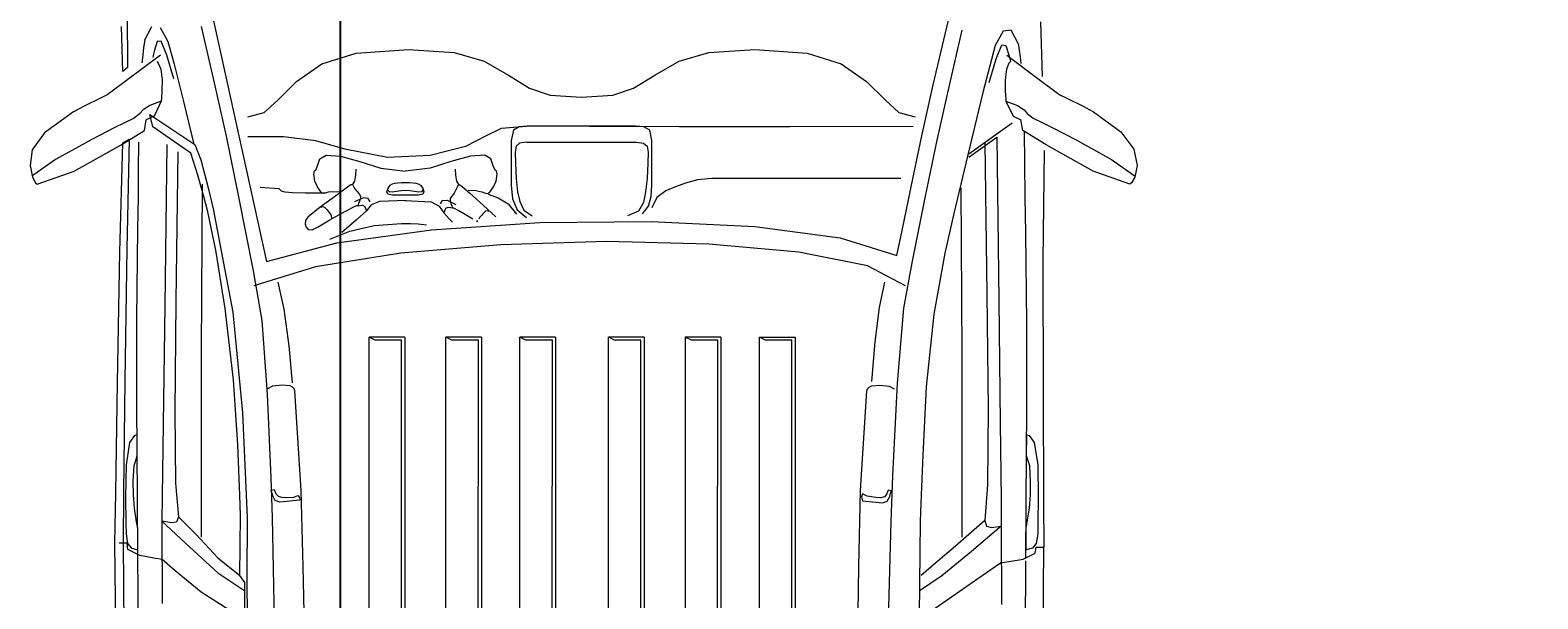
# Model space of a CAD drawing. Units: inches. Extents: x -4347 to -3836, y 955 to 1521.
# Tile 4 of 11: x -4133 to -4072, y 1065 to 1088. Entities that reach past the tile are written whole.
import ezdxf

# ---------------------------------------------------------------- set-up
doc = ezdxf.new("R2010")
doc.units = ezdxf.units.IN
doc.header["$MEASUREMENT"] = 0
doc.layers.add('A-ANNO-DIMS', color=2, linetype='Continuous', lineweight=18)
doc.layers.add('A-SITE-VEHC', color=8, linetype='Continuous', lineweight=13)
doc.styles.get("Standard").update_dxf_attribs({"font": 'arial.ttf'})
doc.dimstyles.get("Standard").update_dxf_attribs({"dimtxt": 0.18, "dimasz": 0.18, "dimexe": 0.18, "dimexo": 0.0625, "dimgap": 0.09, "dimtad": 0, "dimtih": 1, "dimtoh": 1, "dimdec": 0, "dimzin": 0, "dimdsep": 46, "dimlunit": 3, "dimtxsty": 'Standard', "dimcen": 0.09, "dimadec": 0, "dimazin": 0, "dimtfac": 1, "dimtdec": 0, "dimtofl": 0, "dimtmove": 0, "dimatfit": 3, "dimfxl": 1, "dimtolj": 1, "dimtzin": 0, "dimarcsym": 0})

# ---------------------------------------------------------------- blocks, each defined once
blk = doc.blocks.new('*D47')
at = {"layer": 'A-ANNO-DIMS', "color": 0, "lineweight": -2, "transparency": 16777216}
for p, q in [((-4120.58, 1288.726), (-4120.58, 966.959)), ((-3940.58, 1288.726), (-3940.58, 966.959)), ((-4120.4, 967.139), (-4030.97, 967.139)), ((-3940.76, 967.139), (-4030.189, 967.139))]:
    blk.add_line(p, q, dxfattribs=at)
at = {"layer": 'A-ANNO-DIMS', "color": 0, "transparency": 16777216}
for points in [[(-4120.4, 967.169), (-4120.4, 967.109), (-4120.58, 967.139)], [(-3940.76, 967.169), (-3940.76, 967.109), (-3940.58, 967.139)]]:
    blk.add_solid(points, dxfattribs=at)
at = {"layer": 'Defpoints', "color": 0, "transparency": 16777216}
for p in [(-4120.58, 1288.789), (-3940.58, 1288.789), (-3940.58, 967.139)]:
    blk.add_point(p, dxfattribs=at)
at = {"layer": 'A-ANNO-DIMS', "color": 0, "transparency": 16777216, "insert": (-4030.58, 967.139), "char_height": 0.18, "attachment_point": 5}
blk.add_mtext('\\A1;15\'-0"', dxfattribs=at)

msp = doc.modelspace()

# ---------------------------------------------------------------- linework, layer by layer
at = {"layer": 'A-SITE-VEHC'}
for p, q in [((-4125.796, 1088.55), (-4123.555, 1078.317)), ((-4096.245, 1087.523), (-4096.02, 1088.485)), ((-4129.327, 1085.96), (-4129.374, 1087.772)), ((-4129.151, 1088.327), (-4129.134, 1086.126)), ((-4128.446, 1087.238), (-4128.158, 1087.781)), ((-4126.173, 1087.783), (-4125.652, 1085.508)), ((-4092.424, 1087.964), (-4092.357, 1085.761)), ((-4128.446, 1087.238), (-4128.489, 1086.935)), ((-4127.947, 1087.167), (-4128.057, 1086.827)), ((-4127.78, 1087.191), (-4127.947, 1087.167)), ((-4127.831, 1087.739), (-4127.52, 1087.167)), ((-4127.557, 1086.621), (-4127.78, 1087.191)), ((-4127.52, 1087.167), (-4127.264, 1086.261)), ((-4096.732, 1085.425), (-4096.245, 1087.523)), ((-4095.586, 1087.631), (-4096.106, 1085.355)), ((-4093.927, 1087.587), (-4094.239, 1087.015)), ((-4093.601, 1087.629), (-4093.927, 1087.587)), ((-4093.313, 1087.086), (-4093.601, 1087.629)), ((-4127.818, 1086.623), (-4129.178, 1085.607)), ((-4128.526, 1086.625), (-4128.559, 1086.31)), ((-4128.489, 1086.935), (-4128.526, 1086.625)), ((-4128.111, 1086.606), (-4128.125, 1086.526)), ((-4128.057, 1086.827), (-4128.111, 1086.606)), ((-4127.271, 1085.672), (-4127.557, 1086.621)), ((-4121.318, 1086.274), (-4119.947, 1086.708)), ((-4119.947, 1086.708), (-4117.842, 1086.856)), ((-4117.842, 1086.856), (-4115.997, 1086.731)), ((-4115.997, 1086.731), (-4114.794, 1086.375)), ((-4106.959, 1086.375), (-4105.756, 1086.731)), ((-4105.756, 1086.731), (-4103.911, 1086.856)), ((-4103.911, 1086.856), (-4101.806, 1086.708)), ((-4101.806, 1086.708), (-4100.435, 1086.274)), ((-4094.239, 1087.015), (-4094.743, 1085.127)), ((-4094.202, 1086.469), (-4093.979, 1087.039)), ((-4093.979, 1087.039), (-4093.811, 1087.015)), ((-4093.811, 1087.015), (-4093.702, 1086.675)), ((-4093.776, 1086.623), (-4092.415, 1085.607)), ((-4093.702, 1086.675), (-4093.648, 1086.453)), ((-4093.313, 1087.086), (-4093.275, 1086.823)), ((-4093.275, 1086.823), (-4093.242, 1086.554)), ((-4093.242, 1086.554), (-4093.212, 1086.282)), ((-4129.134, 1086.126), (-4129.327, 1085.96)), ((-4127.96, 1086.374), (-4127.905, 1086.299)), ((-4127.905, 1086.299), (-4127.802, 1086.058)), ((-4127.802, 1086.058), (-4127.746, 1085.627)), ((-4127.264, 1086.261), (-4126.888, 1084.763)), ((-4122.337, 1085.565), (-4121.318, 1086.274)), ((-4114.794, 1086.375), (-4113.815, 1085.812)), ((-4107.938, 1085.812), (-4106.959, 1086.375)), ((-4100.435, 1086.274), (-4099.416, 1085.565)), ((-4094.488, 1085.52), (-4094.202, 1086.469)), ((-4093.792, 1086.058), (-4093.847, 1085.627)), ((-4093.689, 1086.299), (-4093.792, 1086.058)), ((-4093.634, 1086.374), (-4093.689, 1086.299)), ((-4093.648, 1086.453), (-4093.634, 1086.374)), ((-4129.178, 1085.607), (-4129.803, 1085.137)), ((-4127.746, 1085.627), (-4127.756, 1085.168)), ((-4125.652, 1085.508), (-4125.171, 1083.359)), ((-4123.093, 1084.819), (-4122.337, 1085.565)), ((-4113.815, 1085.812), (-4112.968, 1085.291)), ((-4108.785, 1085.291), (-4107.938, 1085.812)), ((-4099.416, 1085.565), (-4098.66, 1084.819)), ((-4097.194, 1083.372), (-4096.732, 1085.425)), ((-4096.106, 1085.355), (-4096.588, 1083.207)), ((-4093.847, 1085.627), (-4093.838, 1085.168)), ((-4092.415, 1085.607), (-4091.791, 1085.137)), ((-4130.255, 1084.876), (-4130.857, 1084.58)), ((-4129.953, 1085.022), (-4130.255, 1084.876)), ((-4129.803, 1085.137), (-4129.953, 1085.022)), ((-4127.782, 1084.773), (-4128.241, 1084.596)), ((-4127.782, 1084.773), (-4128.067, 1084.168)), ((-4127.773, 1084.876), (-4127.782, 1084.773)), ((-4127.756, 1085.168), (-4127.773, 1084.876)), ((-4126.888, 1084.763), (-4126.474, 1083.045)), ((-4123.637, 1084.319), (-4123.093, 1084.819)), ((-4112.968, 1085.291), (-4112.139, 1085.015)), ((-4112.139, 1085.015), (-4110.876, 1084.933)), ((-4110.876, 1084.933), (-4109.614, 1085.015)), ((-4109.614, 1085.015), (-4108.785, 1085.291)), ((-4098.66, 1084.819), (-4098.116, 1084.319)), ((-4094.743, 1085.127), (-4095.43, 1082.282)), ((-4093.838, 1085.168), (-4093.821, 1084.876)), ((-4093.821, 1084.876), (-4093.811, 1084.773)), ((-4093.811, 1084.773), (-4093.527, 1084.168)), ((-4093.811, 1084.773), (-4093.353, 1084.596)), ((-4091.791, 1085.137), (-4091.64, 1085.022)), ((-4091.64, 1085.022), (-4091.338, 1084.876)), ((-4091.338, 1084.876), (-4090.736, 1084.581)), ((-4131.306, 1084.346), (-4132.479, 1083.5)), ((-4130.857, 1084.58), (-4131.306, 1084.346)), ((-4128.636, 1084.274), (-4128.872, 1084.095)), ((-4128.51, 1084.427), (-4128.636, 1084.274)), ((-4128.241, 1084.596), (-4128.51, 1084.427)), ((-4128.067, 1084.168), (-4128.387, 1084.025)), ((-4128.238, 1084.237), (-4126.432, 1083.024)), ((-4128.114, 1083.741), (-4128.238, 1084.237)), ((-4124.296, 1084.146), (-4123.637, 1084.319)), ((-4098.116, 1084.319), (-4097.457, 1084.146)), ((-4093.527, 1084.168), (-4093.206, 1084.025)), ((-4093.353, 1084.596), (-4093.084, 1084.427)), ((-4093.084, 1084.427), (-4092.957, 1084.274)), ((-4092.957, 1084.274), (-4092.721, 1084.095)), ((-4090.736, 1084.581), (-4090.288, 1084.346)), ((-4090.288, 1084.346), (-4089.195, 1083.54)), ((-4129.669, 1083.705), (-4130.575, 1083.232)), ((-4129.29, 1083.884), (-4129.669, 1083.705)), ((-4129.394, 1083.015), (-4128.458, 1083.598)), ((-4128.872, 1084.095), (-4129.29, 1083.884)), ((-4128.458, 1083.598), (-4128.387, 1084.025)), ((-4126.597, 1082.679), (-4128.114, 1083.741)), ((-4114.105, 1083.666), (-4114.709, 1083.381)), ((-4112.922, 1083.762), (-4114.105, 1083.666)), ((-4113.616, 1083.6), (-4113.705, 1083.193)), ((-4113.385, 1083.743), (-4113.616, 1083.6)), ((-4113.064, 1083.76), (-4113.385, 1083.743)), ((-4108.689, 1083.76), (-4113.064, 1083.76)), ((-4110.555, 1083.749), (-4112.922, 1083.762)), ((-4106.958, 1083.742), (-4110.555, 1083.749)), ((-4108.368, 1083.743), (-4108.689, 1083.76)), ((-4108.137, 1083.6), (-4108.368, 1083.743)), ((-4108.048, 1083.193), (-4108.137, 1083.6)), ((-4102.499, 1083.742), (-4106.958, 1083.742)), ((-4097.542, 1083.755), (-4102.499, 1083.742)), ((-4093.562, 1083.883), (-4095.306, 1082.637)), ((-4093.135, 1083.598), (-4093.206, 1084.025)), ((-4092.2, 1083.015), (-4093.135, 1083.598)), ((-4093.077, 1083.58), (-4093.063, 1082.284)), ((-4092.721, 1084.095), (-4092.303, 1083.884)), ((-4092.303, 1083.884), (-4091.925, 1083.705)), ((-4091.925, 1083.705), (-4091.018, 1083.232)), ((-4089.195, 1083.54), (-4088.662, 1082.837)), ((-4132.479, 1083.5), (-4132.972, 1082.817)), ((-4130.575, 1083.232), (-4132.028, 1082.422)), ((-4131.288, 1081.951), (-4129.394, 1083.015)), ((-4129.441, 1078.695), (-4129.327, 1083.093)), ((-4129.327, 1083.093), (-4129.065, 1083.25)), ((-4129.065, 1083.25), (-4129.168, 1078.829)), ((-4128.695, 1083.124), (-4128.707, 1081.983)), ((-4127.551, 1083.035), (-4127.643, 1076.536)), ((-4126.432, 1083.024), (-4126.19, 1082.409)), ((-4125.171, 1083.359), (-4124.669, 1080.929)), ((-4122.866, 1083.341), (-4124.294, 1083.341)), ((-4121.564, 1083.176), (-4122.866, 1083.341)), ((-4120.394, 1082.845), (-4121.564, 1083.176)), ((-4115.541, 1082.955), (-4116.969, 1082.584)), ((-4114.709, 1083.381), (-4115.541, 1082.955)), ((-4113.705, 1083.193), (-4113.705, 1081.399)), ((-4113.512, 1082.958), (-4113.549, 1082.726)), ((-4113.37, 1083.083), (-4113.512, 1082.958)), ((-4113.082, 1083.12), (-4113.37, 1083.083)), ((-4113.082, 1083.12), (-4108.67, 1083.12)), ((-4108.67, 1083.12), (-4108.383, 1083.083)), ((-4108.383, 1083.083), (-4108.241, 1082.958)), ((-4108.241, 1082.958), (-4108.204, 1082.726)), ((-4108.048, 1081.399), (-4108.048, 1083.193)), ((-4097.557, 1081.651), (-4097.194, 1083.372)), ((-4096.588, 1083.207), (-4097.06, 1080.944)), ((-4095.299, 1082.514), (-4094.184, 1083.321)), ((-4094.666, 1083.1), (-4094.575, 1077.006)), ((-4094.184, 1083.321), (-4094.095, 1076.748)), ((-4090.306, 1081.951), (-4092.2, 1083.015)), ((-4091.018, 1083.232), (-4089.565, 1082.422)), ((-4132.972, 1082.817), (-4133.054, 1082.186)), ((-4132.028, 1082.422), (-4132.983, 1081.759)), ((-4127.109, 1082.732), (-4127.197, 1076.72)), ((-4126.306, 1081.79), (-4126.597, 1082.679)), ((-4126.19, 1082.409), (-4125.892, 1081.291)), ((-4121.495, 1082.177), (-4121.402, 1082.455)), ((-4121.402, 1082.455), (-4121.154, 1082.6)), ((-4121.154, 1082.6), (-4120.579, 1082.561)), ((-4120.579, 1082.561), (-4119.791, 1082.34)), ((-4118.684, 1082.501), (-4120.394, 1082.845)), ((-4119.791, 1082.34), (-4118.951, 1082.081)), ((-4116.969, 1082.584), (-4118.684, 1082.501)), ((-4116.132, 1082.34), (-4116.971, 1082.081)), ((-4115.343, 1082.561), (-4116.132, 1082.34)), ((-4114.768, 1082.6), (-4115.343, 1082.561)), ((-4114.521, 1082.455), (-4114.768, 1082.6)), ((-4114.428, 1082.177), (-4114.521, 1082.455)), ((-4113.549, 1082.726), (-4113.539, 1082.274)), ((-4108.204, 1082.726), (-4108.213, 1082.274)), ((-4092.271, 1082.79), (-4092.321, 1078.342)), ((-4089.565, 1082.422), (-4088.611, 1081.759)), ((-4088.662, 1082.837), (-4088.54, 1082.186)), ((-4133.054, 1082.186), (-4132.964, 1081.708)), ((-4132.964, 1081.708), (-4132.835, 1081.49)), ((-4132.769, 1081.439), (-4131.288, 1081.951)), ((-4128.707, 1081.983), (-4128.71, 1080.917)), ((-4126.064, 1080.931), (-4126.306, 1081.79)), ((-4121.65, 1081.829), (-4121.618, 1081.972)), ((-4121.608, 1081.554), (-4121.65, 1081.829)), ((-4121.618, 1081.972), (-4121.563, 1082.003)), ((-4121.563, 1082.003), (-4121.495, 1082.177)), ((-4119.967, 1081.793), (-4120.005, 1081.557)), ((-4119.957, 1082.039), (-4119.967, 1081.793)), ((-4118.951, 1082.081), (-4117.961, 1081.957)), ((-4116.971, 1082.081), (-4117.961, 1081.957)), ((-4115.966, 1082.039), (-4115.954, 1081.794)), ((-4115.954, 1081.794), (-4115.914, 1081.559)), ((-4114.359, 1082.003), (-4114.428, 1082.177)), ((-4114.305, 1081.972), (-4114.359, 1082.003)), ((-4114.314, 1081.554), (-4114.272, 1081.829)), ((-4114.272, 1081.829), (-4114.305, 1081.972)), ((-4113.539, 1082.274), (-4113.507, 1081.661)), ((-4108.213, 1082.274), (-4108.246, 1081.661)), ((-4095.43, 1082.282), (-4095.911, 1080.252)), ((-4093.063, 1082.284), (-4093.052, 1080.914)), ((-4088.825, 1081.439), (-4090.306, 1081.951)), ((-4088.63, 1081.708), (-4088.759, 1081.49)), ((-4088.54, 1082.186), (-4088.63, 1081.708)), ((-4132.835, 1081.49), (-4132.769, 1081.439)), ((-4126.132, 1081.437), (-4126.174, 1074.715)), ((-4125.892, 1081.291), (-4125.687, 1080.444)), ((-4123.041, 1081.246), (-4123.798, 1081.301)), ((-4123.019, 1081.216), (-4123.041, 1081.246)), ((-4122.943, 1081.156), (-4123.019, 1081.216)), ((-4122.793, 1081.108), (-4122.943, 1081.156)), ((-4122.5, 1081.086), (-4122.793, 1081.108)), ((-4121.497, 1081.32), (-4121.608, 1081.554)), ((-4121.394, 1081.161), (-4121.497, 1081.32)), ((-4121.327, 1081.08), (-4121.394, 1081.161)), ((-4121.07, 1081.105), (-4121.183, 1081.069)), ((-4120.89, 1081.127), (-4121.07, 1081.105)), ((-4120.607, 1081.115), (-4120.89, 1081.127)), ((-4120.241, 1081.353), (-4120.673, 1081.034)), ((-4120.151, 1081.411), (-4120.241, 1081.353)), ((-4120.116, 1081.412), (-4120.151, 1081.411)), ((-4120.11, 1081.401), (-4120.116, 1081.412)), ((-4120.005, 1081.557), (-4120.11, 1081.401)), ((-4120.073, 1081.399), (-4120.007, 1081.259)), ((-4120.007, 1081.259), (-4119.917, 1081.147)), ((-4119.917, 1081.147), (-4119.825, 1081.048)), ((-4118.706, 1081.122), (-4118.657, 1081.271)), ((-4118.663, 1081.029), (-4118.706, 1081.122)), ((-4118.663, 1081.196), (-4118.657, 1081.271)), ((-4118.608, 1081.129), (-4118.663, 1081.196)), ((-4118.657, 1081.271), (-4118.569, 1081.396)), ((-4118.492, 1081.115), (-4118.608, 1081.129)), ((-4118.569, 1081.396), (-4118.476, 1081.45)), ((-4118.326, 1081.144), (-4118.492, 1081.115)), ((-4118.476, 1081.45), (-4118.382, 1081.472)), ((-4118.382, 1081.472), (-4118.267, 1081.487)), ((-4118.137, 1081.169), (-4118.326, 1081.144)), ((-4118.267, 1081.487), (-4118.119, 1081.496)), ((-4117.952, 1081.179), (-4118.137, 1081.169)), ((-4118.119, 1081.496), (-4117.961, 1081.499)), ((-4117.961, 1081.499), (-4117.803, 1081.496)), ((-4117.772, 1081.169), (-4117.952, 1081.179)), ((-4117.803, 1081.496), (-4117.656, 1081.487)), ((-4117.592, 1081.144), (-4117.772, 1081.169)), ((-4117.656, 1081.487), (-4117.54, 1081.472)), ((-4117.43, 1081.115), (-4117.592, 1081.144)), ((-4117.54, 1081.472), (-4117.447, 1081.45)), ((-4117.447, 1081.45), (-4117.353, 1081.396)), ((-4117.314, 1081.129), (-4117.43, 1081.115)), ((-4117.353, 1081.396), (-4117.266, 1081.271)), ((-4117.26, 1081.196), (-4117.314, 1081.129)), ((-4117.266, 1081.271), (-4117.217, 1081.122)), ((-4117.266, 1081.271), (-4117.26, 1081.196)), ((-4117.217, 1081.122), (-4117.26, 1081.029)), ((-4115.915, 1081.234), (-4116.001, 1081.073)), ((-4115.847, 1081.399), (-4115.915, 1081.234)), ((-4115.914, 1081.559), (-4115.81, 1081.399)), ((-4115.81, 1081.399), (-4115.803, 1081.409)), ((-4115.803, 1081.409), (-4115.768, 1081.407)), ((-4115.768, 1081.407), (-4115.682, 1081.344)), ((-4115.682, 1081.344), (-4115.369, 1081.065)), ((-4115.444, 1081.188), (-4115.127, 1081.182)), ((-4115.127, 1081.182), (-4114.885, 1081.124)), ((-4114.885, 1081.124), (-4114.739, 1081.069)), ((-4114.596, 1081.08), (-4114.529, 1081.161)), ((-4114.529, 1081.161), (-4114.426, 1081.32)), ((-4114.426, 1081.32), (-4114.314, 1081.554)), ((-4113.705, 1081.399), (-4113.657, 1080.844)), ((-4113.507, 1081.661), (-4113.449, 1081.124)), ((-4113.449, 1081.124), (-4113.367, 1080.739)), ((-4108.304, 1081.124), (-4108.391, 1080.702)), ((-4108.246, 1081.661), (-4108.304, 1081.124)), ((-4108.079, 1080.94), (-4108.048, 1081.399)), ((-4107.492, 1081.162), (-4107.852, 1080.901)), ((-4107.105, 1081.328), (-4107.492, 1081.162)), ((-4106.701, 1081.475), (-4107.105, 1081.328)), ((-4106.212, 1081.604), (-4106.701, 1081.475)), ((-4105.643, 1081.659), (-4106.212, 1081.604)), ((-4098.033, 1081.659), (-4105.643, 1081.659)), ((-4097.988, 1079.571), (-4097.557, 1081.651)), ((-4095.627, 1081.285), (-4095.586, 1074.603)), ((-4088.759, 1081.49), (-4088.825, 1081.439)), ((-4128.71, 1080.917), (-4128.73, 1079.622)), ((-4125.908, 1080.322), (-4126.064, 1080.931)), ((-4124.669, 1080.929), (-4124.085, 1077.944)), ((-4121.979, 1081.073), (-4122.5, 1081.086)), ((-4121.183, 1081.069), (-4121.979, 1081.073)), ((-4121.387, 1080.509), (-4121.881, 1080.111)), ((-4120.673, 1081.034), (-4121.387, 1080.509)), ((-4121.356, 1080.514), (-4121.285, 1080.534)), ((-4121.262, 1081.052), (-4121.327, 1081.08)), ((-4121.285, 1080.534), (-4121.212, 1080.51)), ((-4121.183, 1081.069), (-4121.262, 1081.052)), ((-4121.212, 1080.51), (-4121.122, 1080.419)), ((-4120.397, 1080.338), (-4119.932, 1080.577)), ((-4119.643, 1080.883), (-4120.006, 1080.727)), ((-4119.932, 1080.577), (-4119.919, 1080.572)), ((-4119.919, 1080.572), (-4119.875, 1080.568)), ((-4119.875, 1080.568), (-4119.794, 1080.579)), ((-4119.857, 1080.601), (-4119.858, 1080.582)), ((-4119.845, 1080.657), (-4119.857, 1080.601)), ((-4119.803, 1080.753), (-4119.845, 1080.657)), ((-4119.825, 1081.048), (-4119.767, 1080.955)), ((-4119.762, 1080.86), (-4119.803, 1080.753)), ((-4119.794, 1080.579), (-4119.688, 1080.59)), ((-4119.767, 1080.955), (-4119.762, 1080.86)), ((-4119.688, 1080.59), (-4119.591, 1080.539)), ((-4119.456, 1080.857), (-4119.643, 1080.883)), ((-4119.591, 1080.539), (-4119.531, 1080.363)), ((-4119.339, 1080.606), (-4119.531, 1080.363)), ((-4119.383, 1080.722), (-4119.456, 1080.857)), ((-4118.999, 1080.737), (-4119.339, 1080.606)), ((-4117.934, 1080.776), (-4118.999, 1080.737)), ((-4118.492, 1080.996), (-4118.663, 1081.029)), ((-4117.43, 1080.996), (-4118.492, 1080.996)), ((-4117.989, 1080.776), (-4116.928, 1080.719)), ((-4117.26, 1081.029), (-4117.43, 1080.996)), ((-4116.928, 1080.719), (-4116.599, 1080.552)), ((-4116.599, 1080.552), (-4116.423, 1080.282)), ((-4116.552, 1080.648), (-4116.472, 1080.779)), ((-4116.472, 1080.779), (-4116.284, 1080.795)), ((-4116.255, 1080.5), (-4116.354, 1080.454)), ((-4116.284, 1080.795), (-4115.929, 1080.621)), ((-4116.149, 1080.483), (-4116.255, 1080.5)), ((-4116.156, 1080.86), (-4116.166, 1080.766)), ((-4116.166, 1080.766), (-4116.131, 1080.657)), ((-4116.094, 1080.95), (-4116.156, 1080.86)), ((-4116.131, 1080.657), (-4116.094, 1080.559)), ((-4116.001, 1081.073), (-4116.094, 1080.95)), ((-4116.094, 1080.559), (-4116.085, 1080.502)), ((-4116.085, 1080.502), (-4116.085, 1080.483)), ((-4115.369, 1081.065), (-4114.822, 1080.576)), ((-4114.822, 1080.576), (-4114.32, 1080.113)), ((-4114.739, 1081.069), (-4114.66, 1081.052)), ((-4114.66, 1081.052), (-4114.596, 1081.08)), ((-4114.631, 1081.025), (-4114.234, 1080.879)), ((-4114.234, 1080.879), (-4113.825, 1080.647)), ((-4113.825, 1080.647), (-4113.501, 1080.226)), ((-4113.657, 1080.844), (-4113.474, 1080.395)), ((-4113.367, 1080.739), (-4113.198, 1080.387)), ((-4108.391, 1080.702), (-4108.591, 1080.346)), ((-4108.422, 1080.245), (-4108.192, 1080.546)), ((-4108.192, 1080.546), (-4108.079, 1080.94)), ((-4107.852, 1080.901), (-4108.056, 1080.487)), ((-4097.06, 1080.944), (-4097.594, 1078.27)), ((-4093.052, 1080.914), (-4093.028, 1079.469)), ((-4125.589, 1078.782), (-4125.908, 1080.322)), ((-4125.687, 1080.444), (-4124.902, 1076.285)), ((-4121.978, 1079.966), (-4121.999, 1079.827)), ((-4121.881, 1080.111), (-4121.978, 1079.966)), ((-4121.471, 1079.713), (-4121.004, 1080.001)), ((-4121.122, 1080.419), (-4121.022, 1080.289)), ((-4121.022, 1080.289), (-4120.947, 1080.166)), ((-4121.004, 1080.001), (-4120.397, 1080.338)), ((-4120.947, 1080.166), (-4120.931, 1080.052)), ((-4119.926, 1080.003), (-4120.335, 1079.652)), ((-4119.531, 1080.363), (-4119.926, 1080.003)), ((-4116.909, 1079.6), (-4112.556, 1079.889)), ((-4116.354, 1080.454), (-4116.423, 1080.282)), ((-4116.423, 1080.282), (-4116.316, 1080.164)), ((-4116.316, 1080.164), (-4116.206, 1080.043)), ((-4116.206, 1080.043), (-4116.075, 1079.9)), ((-4116.069, 1080.469), (-4116.149, 1080.483)), ((-4116.025, 1080.471), (-4116.069, 1080.469)), ((-4116.012, 1080.474), (-4116.025, 1080.471)), ((-4115.816, 1080.365), (-4116.012, 1080.474)), ((-4115.556, 1080.211), (-4115.816, 1080.365)), ((-4115.251, 1080.023), (-4115.556, 1080.211)), ((-4115.105, 1079.936), (-4115.053, 1079.94)), ((-4115.088, 1079.938), (-4115.105, 1079.936)), ((-4115.071, 1079.939), (-4115.088, 1079.938)), ((-4115.053, 1079.94), (-4115.071, 1079.939)), ((-4114.963, 1080.099), (-4115.012, 1080.024)), ((-4114.9, 1080.175), (-4114.963, 1080.099)), ((-4114.831, 1080.254), (-4114.9, 1080.175)), ((-4114.736, 1080.341), (-4114.831, 1080.254)), ((-4114.663, 1080.36), (-4114.736, 1080.341)), ((-4114.593, 1080.337), (-4114.663, 1080.36)), ((-4113.474, 1080.395), (-4113.095, 1080.097)), ((-4113.198, 1080.387), (-4112.865, 1080.155)), ((-4112.556, 1079.889), (-4108.083, 1079.936)), ((-4108.591, 1080.346), (-4109.037, 1080.161)), ((-4108.083, 1079.936), (-4103.915, 1079.734)), ((-4095.911, 1080.252), (-4096.269, 1078.657)), ((-4128.73, 1079.622), (-4128.771, 1076.014)), ((-4121.999, 1079.827), (-4121.958, 1079.702)), ((-4121.958, 1079.702), (-4121.869, 1079.607)), ((-4121.869, 1079.607), (-4121.718, 1079.59)), ((-4121.718, 1079.59), (-4121.471, 1079.713)), ((-4120.998, 1079.225), (-4120.201, 1079.543)), ((-4120.717, 1079.074), (-4116.909, 1079.6)), ((-4120.335, 1079.652), (-4120.524, 1079.495)), ((-4120.201, 1079.543), (-4119.214, 1079.767)), ((-4119.214, 1079.767), (-4118.117, 1079.852)), ((-4118.117, 1079.852), (-4117.763, 1079.851)), ((-4117.763, 1079.851), (-4117.449, 1079.838)), ((-4117.449, 1079.838), (-4117.12, 1079.8)), ((-4103.915, 1079.734), (-4100.478, 1079.277)), ((-4100.478, 1079.277), (-4098.197, 1078.561)), ((-4098.197, 1078.561), (-4097.988, 1079.571)), ((-4093.028, 1079.469), (-4092.988, 1075.861)), ((-4129.542, 1073.458), (-4129.441, 1078.695)), ((-4129.168, 1078.829), (-4129.245, 1073.537)), ((-4125.206, 1076.426), (-4125.589, 1078.782)), ((-4123.555, 1078.317), (-4120.717, 1079.074)), ((-4114.126, 1078.997), (-4118.148, 1078.657)), ((-4109.877, 1079.12), (-4114.126, 1078.997)), ((-4105.761, 1079.022), (-4109.877, 1079.12)), ((-4102.143, 1078.697), (-4105.761, 1079.022)), ((-4099.384, 1078.141), (-4102.143, 1078.697)), ((-4121.578, 1078.105), (-4124.056, 1077.348)), ((-4118.148, 1078.657), (-4121.578, 1078.105)), ((-4097.846, 1077.348), (-4099.384, 1078.141)), ((-4097.594, 1078.27), (-4097.931, 1076.442)), ((-4096.269, 1078.657), (-4096.705, 1076.2)), ((-4092.321, 1078.342), (-4092.319, 1073.075)), ((-4124.085, 1077.944), (-4123.737, 1075.946)), ((-4123.096, 1077.496), (-4122.854, 1076.402)), ((-4098.689, 1077.496), (-4098.912, 1076.472)), ((-4094.575, 1077.006), (-4094.532, 1072.391)), ((-4127.643, 1076.536), (-4127.706, 1071.784)), ((-4127.197, 1076.72), (-4127.235, 1072.283)), ((-4124.874, 1073.567), (-4125.206, 1076.426)), ((-4124.902, 1076.285), (-4124.509, 1072.233)), ((-4122.854, 1076.402), (-4122.649, 1074.932)), ((-4098.912, 1076.472), (-4099.088, 1075.083)), ((-4097.931, 1076.442), (-4098.184, 1073.428)), ((-4094.095, 1076.748), (-4094.039, 1071.829)), ((-4128.771, 1076.014), (-4128.772, 1072.445)), ((-4123.737, 1075.946), (-4123.516, 1072.983)), ((-4096.705, 1076.2), (-4097.015, 1073.277)), ((-4092.988, 1075.861), (-4092.986, 1072.293)), ((-4119.179, 1075.163), (-4119.422, 1075.281)), ((-4117.987, 1075.281), (-4119.422, 1075.281)), ((-4119.421, 1037.674), (-4119.421, 1075.281)), ((-4118.117, 1075.163), (-4119.179, 1075.163)), ((-4118.131, 1038.272), (-4118.117, 1075.163)), ((-4117.988, 1075.281), (-4117.988, 1037.674)), ((-4117.987, 1075.281), (-4117.987, 1037.674)), ((-4116.09, 1075.163), (-4116.334, 1075.281)), ((-4114.899, 1075.281), (-4116.334, 1075.281)), ((-4116.333, 1037.674), (-4116.333, 1075.281)), ((-4115.029, 1075.163), (-4116.09, 1075.163)), ((-4115.043, 1038.272), (-4115.029, 1075.163)), ((-4114.9, 1075.281), (-4114.9, 1037.674)), ((-4114.899, 1075.281), (-4114.899, 1037.674)), ((-4113.113, 1075.163), (-4113.356, 1075.281)), ((-4111.921, 1075.281), (-4113.356, 1075.281)), ((-4113.355, 1037.674), (-4113.355, 1075.281)), ((-4112.051, 1075.163), (-4113.113, 1075.163)), ((-4112.065, 1038.272), (-4112.051, 1075.163)), ((-4111.923, 1075.281), (-4111.923, 1037.674)), ((-4111.921, 1075.281), (-4111.921, 1037.674)), ((-4109.55, 1075.163), (-4109.794, 1075.281)), ((-4108.359, 1075.281), (-4109.794, 1075.281)), ((-4109.792, 1037.674), (-4109.792, 1075.281)), ((-4108.489, 1075.163), (-4109.55, 1075.163)), ((-4108.503, 1038.272), (-4108.489, 1075.163)), ((-4108.36, 1075.281), (-4108.36, 1037.674)), ((-4108.359, 1075.281), (-4108.359, 1037.674)), ((-4106.462, 1075.163), (-4106.706, 1075.281)), ((-4105.271, 1075.281), (-4106.706, 1075.281)), ((-4106.704, 1037.674), (-4106.704, 1075.281)), ((-4105.401, 1075.163), (-4106.462, 1075.163)), ((-4105.415, 1038.272), (-4105.401, 1075.163)), ((-4105.272, 1075.281), (-4105.272, 1037.674)), ((-4105.271, 1075.281), (-4105.271, 1037.674)), ((-4103.727, 1037.674), (-4103.727, 1075.281)), ((-4103.483, 1075.163), (-4103.727, 1075.281)), ((-4103.727, 1075.281), (-4102.293, 1075.281)), ((-4102.422, 1075.163), (-4103.483, 1075.163)), ((-4102.436, 1038.272), (-4102.422, 1075.163)), ((-4102.293, 1075.281), (-4102.293, 1037.674)), ((-4099.088, 1075.083), (-4099.219, 1073.498)), ((-4126.174, 1074.715), (-4126.176, 1069.391)), ((-4122.649, 1074.932), (-4122.517, 1073.443)), ((-4095.586, 1074.603), (-4095.584, 1069.352)), ((-4129.614, 1069.013), (-4129.542, 1073.458)), ((-4129.245, 1073.537), (-4129.294, 1069.038)), ((-4124.695, 1070.949), (-4124.874, 1073.567)), ((-4123.313, 1073.305), (-4123.51, 1073.195)), ((-4122.936, 1073.346), (-4123.313, 1073.305)), ((-4122.595, 1073.313), (-4122.936, 1073.346)), ((-4122.508, 1073.27), (-4122.595, 1073.313)), ((-4122.438, 1073.199), (-4122.508, 1073.27)), ((-4099.381, 1073.199), (-4099.31, 1073.27)), ((-4099.31, 1073.27), (-4099.223, 1073.313)), ((-4099.223, 1073.313), (-4098.882, 1073.346)), ((-4098.882, 1073.346), (-4098.506, 1073.305)), ((-4098.506, 1073.305), (-4098.308, 1073.195)), ((-4098.184, 1073.428), (-4098.368, 1069.694)), ((-4097.015, 1073.277), (-4097.158, 1070.529)), ((-4123.516, 1072.983), (-4123.372, 1069.62)), ((-4122.406, 1073.112), (-4122.438, 1073.199)), ((-4122.148, 1069.103), (-4122.406, 1073.112)), ((-4099.661, 1069.103), (-4099.412, 1073.112)), ((-4099.412, 1073.112), (-4099.381, 1073.199)), ((-4092.319, 1073.075), (-4092.295, 1068.676)), ((-4128.772, 1072.445), (-4128.766, 1070.83)), ((-4127.235, 1072.283), (-4127.206, 1069.402)), ((-4124.509, 1072.233), (-4124.329, 1068.022)), ((-4094.532, 1072.391), (-4094.555, 1069.331)), ((-4092.986, 1072.293), (-4092.993, 1070.678)), ((-4127.706, 1071.784), (-4127.743, 1068.866)), ((-4094.039, 1071.829), (-4094.009, 1068.746)), ((-4129.052, 1071.038), (-4129.191, 1070.143)), ((-4128.853, 1071.327), (-4129.052, 1071.038)), ((-4128.752, 1071.347), (-4128.853, 1071.327)), ((-4128.766, 1070.83), (-4128.73, 1066.524)), ((-4128.744, 1070.507), (-4128.752, 1071.347)), ((-4124.616, 1068.922), (-4124.695, 1070.949)), ((-4092.98, 1070.507), (-4092.972, 1071.347)), ((-4092.972, 1071.347), (-4092.871, 1071.327)), ((-4092.871, 1071.327), (-4092.672, 1071.038)), ((-4092.672, 1071.038), (-4092.533, 1070.143)), ((-4128.87, 1070.095), (-4128.744, 1070.507)), ((-4097.158, 1070.529), (-4097.239, 1068.597)), ((-4092.993, 1070.678), (-4093.028, 1066.372)), ((-4092.854, 1070.095), (-4092.98, 1070.507)), ((-4129.191, 1070.143), (-4129.216, 1068.857)), ((-4128.905, 1069.487), (-4128.87, 1070.095)), ((-4123.372, 1069.62), (-4123.32, 1068.019)), ((-4098.368, 1069.694), (-4098.438, 1067.866)), ((-4092.819, 1069.487), (-4092.854, 1070.095)), ((-4092.533, 1070.143), (-4092.509, 1068.857)), ((-4129.643, 1066.995), (-4129.614, 1069.013)), ((-4129.294, 1069.038), (-4129.312, 1066.995)), ((-4128.904, 1068.939), (-4128.905, 1069.487)), ((-4127.206, 1069.402), (-4127.093, 1068.054)), ((-4126.176, 1069.391), (-4126.17, 1067.226)), ((-4123.358, 1069.123), (-4123.235, 1069.149)), ((-4123.3, 1068.896), (-4123.358, 1069.123)), ((-4123.235, 1069.149), (-4123.183, 1069.003)), ((-4123.183, 1069.003), (-4123.084, 1068.881)), ((-4122.068, 1066.049), (-4122.148, 1069.103)), ((-4099.725, 1066.049), (-4099.661, 1069.103)), ((-4099.579, 1068.969), (-4099.621, 1068.855)), ((-4099.392, 1068.874), (-4099.579, 1068.969)), ((-4098.602, 1068.975), (-4098.701, 1068.853)), ((-4098.55, 1069.121), (-4098.602, 1068.975)), ((-4098.427, 1069.096), (-4098.55, 1069.121)), ((-4098.485, 1068.869), (-4098.427, 1069.096)), ((-4095.584, 1069.352), (-4095.591, 1067.226)), ((-4094.555, 1069.331), (-4094.666, 1067.902)), ((-4092.821, 1068.939), (-4092.819, 1069.487)), ((-4129.216, 1068.857), (-4129.202, 1067.8)), ((-4128.857, 1068.397), (-4128.904, 1068.939)), ((-4128.771, 1067.844), (-4128.857, 1068.397)), ((-4127.743, 1068.866), (-4127.755, 1067.874)), ((-4124.598, 1068.108), (-4124.616, 1068.922)), ((-4123.195, 1068.704), (-4123.3, 1068.896)), ((-4123.007, 1068.637), (-4123.195, 1068.704)), ((-4123.084, 1068.881), (-4122.937, 1068.841)), ((-4122.207, 1068.716), (-4123.007, 1068.637)), ((-4122.937, 1068.841), (-4122.768, 1068.832)), ((-4122.768, 1068.832), (-4122.454, 1068.84)), ((-4122.454, 1068.84), (-4122.288, 1068.913)), ((-4122.288, 1068.913), (-4122.226, 1068.821)), ((-4122.226, 1068.821), (-4122.207, 1068.746)), ((-4122.207, 1068.746), (-4122.207, 1068.716)), ((-4099.621, 1068.855), (-4099.599, 1068.74)), ((-4099.599, 1068.74), (-4099.578, 1068.688)), ((-4099.578, 1068.688), (-4098.777, 1068.61)), ((-4099.039, 1068.826), (-4099.392, 1068.874)), ((-4098.848, 1068.813), (-4099.039, 1068.826)), ((-4098.701, 1068.853), (-4098.848, 1068.813)), ((-4098.777, 1068.61), (-4098.59, 1068.677)), ((-4098.59, 1068.677), (-4098.485, 1068.869)), ((-4097.239, 1068.597), (-4097.264, 1067.866)), ((-4094.009, 1068.746), (-4094, 1067.678)), ((-4092.953, 1067.844), (-4092.867, 1068.397)), ((-4092.867, 1068.397), (-4092.821, 1068.939)), ((-4092.509, 1068.857), (-4092.522, 1067.8)), ((-4092.295, 1068.676), (-4092.281, 1066.834)), ((-4129.202, 1067.8), (-4129.189, 1067.362)), ((-4128.725, 1067.591), (-4128.771, 1067.844)), ((-4127.755, 1067.874), (-4126.633, 1066.835)), ((-4127.37, 1067.802), (-4127.755, 1067.874)), ((-4127.755, 1067.874), (-4127.742, 1064.565)), ((-4127.17, 1067.841), (-4127.37, 1067.802)), ((-4127.093, 1068.054), (-4127.17, 1067.841)), ((-4127.093, 1068.054), (-4126.38, 1067.341)), ((-4124.62, 1065.685), (-4124.598, 1068.108)), ((-4124.329, 1068.022), (-4124.346, 1065.547)), ((-4123.32, 1068.019), (-4123.237, 1063.886)), ((-4098.438, 1067.866), (-4098.543, 1063.914)), ((-4097.264, 1067.866), (-4097.297, 1064.092)), ((-4094.666, 1067.902), (-4095.846, 1066.863)), ((-4094.666, 1067.902), (-4094.588, 1067.678)), ((-4092.999, 1067.591), (-4092.953, 1067.844)), ((-4092.522, 1067.8), (-4092.535, 1067.362)), ((-4129.189, 1067.362), (-4129.133, 1066.977)), ((-4128.725, 1066.718), (-4128.725, 1067.591)), ((-4126.38, 1067.341), (-4125.512, 1066.405)), ((-4094, 1067.678), (-4095.202, 1066.659)), ((-4094.588, 1067.678), (-4094.386, 1067.617)), ((-4094.386, 1067.617), (-4094, 1067.678)), ((-4094, 1067.678), (-4093.989, 1064.522)), ((-4092.999, 1066.718), (-4092.999, 1067.591)), ((-4092.535, 1067.362), (-4092.592, 1066.977)), ((-4129.614, 1063.599), (-4129.643, 1066.995)), ((-4129.158, 1066.987), (-4129.478, 1066.995)), ((-4129.312, 1066.995), (-4129.283, 1063.603)), ((-4129.122, 1066.737), (-4129.158, 1066.987)), ((-4129.133, 1066.977), (-4128.984, 1066.787)), ((-4128.645, 1066.489), (-4129.122, 1066.737)), ((-4128.984, 1066.787), (-4128.725, 1066.718)), ((-4126.633, 1066.835), (-4125.505, 1065.791)), ((-4095.846, 1066.863), (-4096.82, 1066.033)), ((-4095.202, 1066.659), (-4096.392, 1065.681)), ((-4093.118, 1066.341), (-4092.637, 1066.585)), ((-4092.74, 1066.787), (-4092.999, 1066.718)), ((-4092.592, 1066.977), (-4092.74, 1066.787)), ((-4092.637, 1066.585), (-4092.601, 1066.834)), ((-4092.601, 1066.834), (-4092.294, 1066.834)), ((-4092.31, 1063.442), (-4092.281, 1066.834)), ((-4128.73, 1066.524), (-4128.703, 1061.321)), ((-4128.076, 1066.388), (-4128.645, 1066.489)), ((-4127.742, 1066.33), (-4128.076, 1066.388)), ((-4127.222, 1065.875), (-4127.742, 1066.33)), ((-4125.512, 1066.405), (-4124.62, 1065.685)), ((-4122.033, 1064.207), (-4122.068, 1066.049)), ((-4099.752, 1064.207), (-4099.725, 1066.049)), ((-4096.82, 1066.033), (-4097.226, 1065.694)), ((-4094.763, 1065.69), (-4094.036, 1066.192)), ((-4094.036, 1066.192), (-4093.697, 1066.246)), ((-4093.697, 1066.246), (-4093.118, 1066.341)), ((-4093.024, 1066.275), (-4093.052, 1061.072)), ((-4126.18, 1065.018), (-4127.222, 1065.875)), ((-4125.505, 1065.791), (-4124.419, 1065.075)), ((-4124.426, 1065.411), (-4124.62, 1065.685)), ((-4124.412, 1063.007), (-4124.426, 1065.411)), ((-4124.346, 1065.547), (-4124.329, 1063.972)), ((-4096.392, 1065.681), (-4097.262, 1065.089)), ((-4096.001, 1064.832), (-4094.763, 1065.69)), ((-4125.067, 1064.303), (-4126.18, 1065.018)), ((-4096.656, 1064.377), (-4096.001, 1064.832))]:
    msp.add_line(p, q, dxfattribs=at)

# ---------------------------------------------------------------- dimensions: what is measured, and where the dimension line sits
at = {"layer": 'A-ANNO-DIMS'}
dim = msp.add_linear_dim(base=(-3940.58, 967.139), p1=(-4120.58, 1288.789), p2=(-3940.58, 1288.789), dimstyle='Standard', override={"dimdec": 1, "dimlfac": 1, "dimrnd": 0, "dimzin": 1, "dimdsep": 46, "dimlunit": 4, "dimfrac": 2}, dxfattribs=at)
dim.commit()
dim.dimension.update_dxf_attribs({"geometry": '*D47', "text_midpoint": (-4030.58, 967.139)})

doc.saveas('drawing.dxf')
